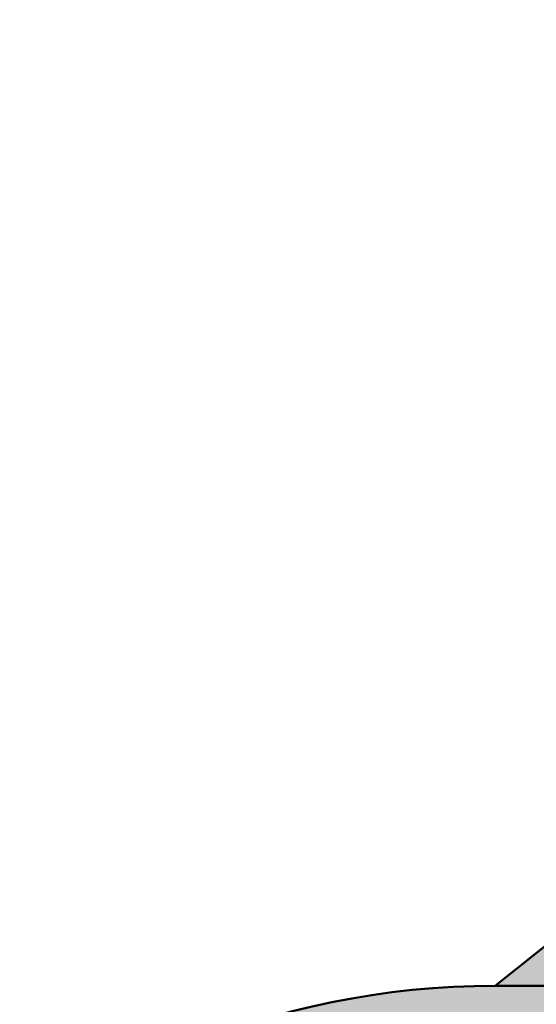
# Model space of a CAD drawing. Units: millimetres. Extents: x 0 to 2267, y 0 to 1823.
# Tile 17 of 256: x 1525.06 to 1531.44, y 1127.19 to 1139.34. Entities that reach past the tile are written whole.
import ezdxf

# ---------------------------------------------------------------- set-up
doc = ezdxf.new("R2010")
doc.units = ezdxf.units.MM
doc.header["$MEASUREMENT"] = 0
for name, color, linetype, lineweight in [('M-DIMS', 2, 'Continuous', 25), ('M-HATC', 252, 'Continuous', 18), ('M-OUTL', 7, 'Continuous', 50)]:
    doc.layers.add(name, color=color, linetype=linetype, lineweight=lineweight)
doc.styles.get("Standard").update_dxf_attribs({"font": 'arial.ttf'})
doc.dimstyles.get("Standard").update_dxf_attribs({"dimtxt": 7, "dimasz": 4, "dimexe": 0.18, "dimexo": 0.0625, "dimgap": 0.09, "dimtad": 0, "dimdec": 0, "dimzin": 0, "dimdsep": 46, "dimtxsty": 'Standard', "dimcen": 0.09, "dimadec": 0, "dimazin": 0, "dimtfac": 1, "dimtdec": 0, "dimtofl": 0, "dimtmove": 0, "dimatfit": 3, "dimfxl": 1, "dimtolj": 1, "dimtzin": 0, "dimarcsym": 0})

# ---------------------------------------------------------------- blocks, each defined once
blk = doc.blocks.new('*D28')
at = {"layer": 'Defpoints', "color": 0, "transparency": 16777216}
for p in [(1523.858, 1124.488), (1530.929, 1117.417)]:
    blk.add_point(p, dxfattribs=at)
at = {"layer": 'M-DIMS', "color": 0, "lineweight": -2, "transparency": 16777216}
for p, q in [((1518.201, 1130.145), (1521.029, 1127.317)), ((1530.929, 1117.327), (1530.929, 1117.507)), ((1530.839, 1117.417), (1531.019, 1117.417))]:
    blk.add_line(p, q, dxfattribs=at)
at = {"layer": 'M-DIMS', "color": 0, "transparency": 16777216}
blk.add_solid([(1521.501, 1127.788), (1520.558, 1126.845), (1523.858, 1124.488)], dxfattribs=at)
at = {"layer": 'M-DIMS', "color": 0, "transparency": 16777216, "insert": (1504.949, 1143.397), "char_height": 7, "attachment_point": 5, "rotation": 314.9998}
blk.add_mtext('\\A1;27X R10', dxfattribs=at)

msp = doc.modelspace()

# ---------------------------------------------------------------- hatches: boundary and pattern name
at = {"layer": 'M-HATC'}
h = msp.add_hatch(color=256, dxfattribs=at)
h.dxf.hatch_style = 1
h.paths.add_polyline_path([(2055.771, 1603.062), (1381.087, 1603.062), (1381.087, 1598.062), (2055.771, 1598.062)])
h.paths.add_polyline_path([(2055.771, 1598.062), (1381.087, 1598.062), (1381.087, 1593.062), (2055.771, 1593.062)])
h.paths.add_polyline_path([(2051.307, 1536.761), (1385.55, 1536.761), (1385.55, 1526.761), (1387.55, 1526.761), (1388.537, 1525.053), (1385.332, 1521.233), (1385.332, 1521.223), (2050.254, 1522.749), (2048.321, 1525.053), (2049.307, 1526.761), (2051.307, 1526.761)])
edge = h.paths.add_edge_path()
edge.add_arc((1847.535, 1379.149), 135, 222.60306, 222.89085, ccw=False)
edge.add_line((1748.166, 1287.766), (1683.092, 1287.766))
edge.add_arc((1583.724, 1379.149), 135, 317.10915, 317.39694, ccw=False)
edge.add_arc((1678.969, 1290.671), 5, 222.8909, 317.1091, ccw=False)
edge.add_arc((1774.213, 1379.149), 135, 222.60306, 222.89085, ccw=False)
edge.add_line((1674.845, 1287.766), (1609.771, 1287.766))
edge.add_arc((1510.403, 1379.149), 135, 317.10915, 317.39694, ccw=False)
edge.add_arc((1605.647, 1290.671), 5, 222.8909, 317.1091, ccw=False)
edge.add_arc((1700.892, 1379.149), 135, 222.60306, 222.89085, ccw=False)
edge.add_line((1601.524, 1287.766), (1536.45, 1287.766))
edge.add_arc((1437.081, 1379.149), 135, 317.10915, 317.39694, ccw=False)
edge.add_arc((1532.326, 1290.671), 5, 222.8909, 317.1091, ccw=False)
edge.add_arc((1627.571, 1379.149), 135, 222.60306, 222.89085, ccw=False)
edge.add_line((1528.203, 1287.766), (1505.929, 1287.766))
edge.add_spline(control_points=[(1505.929, 1287.766), (1504.262, 1287.766), (1504.262, 1282.766), (1505.929, 1282.766)], knot_values=[0, 0, 0, 0, 5, 5, 5, 5], degree=3, periodic=0)
edge.add_line((1505.929, 1282.766), (1930.929, 1282.766))
edge.add_spline(control_points=[(1930.929, 1282.766), (1932.596, 1282.766), (1932.596, 1287.766), (1930.929, 1287.766)], knot_values=[0, 0, 0, 0, 5, 5, 5, 5], degree=3, periodic=0)
edge.add_line((1930.929, 1287.766), (1903.056, 1287.766))
edge.add_arc((1803.688, 1379.149), 135, 317.10915, 317.39694, ccw=False)
edge.add_arc((1898.932, 1290.671), 5, 222.8909, 317.1091, ccw=False)
edge.add_arc((1994.177, 1379.149), 135, 222.60306, 222.89085, ccw=False)
edge.add_line((1894.809, 1287.766), (1829.735, 1287.766))
edge.add_arc((1730.366, 1379.149), 135, 317.10915, 317.39694, ccw=False)
edge.add_arc((1825.611, 1290.671), 5, 222.8909, 317.1091, ccw=False)
edge.add_arc((1920.856, 1379.149), 135, 222.60306, 222.89085, ccw=False)
edge.add_line((1821.487, 1287.766), (1756.413, 1287.766))
edge.add_arc((1657.045, 1379.149), 135, 317.10915, 317.39694, ccw=False)
edge.add_arc((1752.29, 1290.671), 5, 222.8909, 317.1091, ccw=False)
edge = h.paths.add_edge_path()
edge.add_spline(control_points=[(1843.429, 1227.247), (1845.096, 1227.247), (1845.096, 1232.247), (1843.429, 1232.247)], knot_values=[0, 0, 0, 0, 5, 5, 5, 5], degree=3, periodic=0)
edge.add_line((1843.429, 1232.247), (1593.429, 1232.247))
edge.add_spline(control_points=[(1593.429, 1232.247), (1591.762, 1232.247), (1591.762, 1227.247), (1593.429, 1227.247)], knot_values=[0, 0, 0, 0, 5, 5, 5, 5], degree=3, periodic=0)
edge.add_line((1593.429, 1227.247), (1843.429, 1227.247))
h.paths.add_polyline_path([(1905.929, 1127.417), (1530.929, 1127.417, 0.414214), (1520.929, 1117.417), (1530.929, 1117.417), (1915.929, 1117.417, 0.414214)])
edge = h.paths.add_edge_path()
edge.add_arc((1397.086, 1498.408), 12.73, 90.7821, 190.8787, ccw=False)
edge.add_line((1396.912, 1511.136), (1428.01, 1511.349))
edge.add_line((1428.01, 1511.349), (1433.01, 1511.349))
edge.add_line((1433.01, 1511.349), (1434.439, 1511.349))
edge.add_arc((1419.474, 1498.08), 20, 41.561, 74.0821)
edge.add_line((1424.959, 1517.314), (1399.935, 1517.256))
edge.add_spline(control_points=[(1399.931, 1517.256), (1399.884, 1517.213), (1399.833, 1517.169), (1399.777, 1517.124)], knot_values=[11.567499, 11.567499, 11.567499, 11.567499, 11.814249, 11.814249, 11.814249, 11.814249], degree=3, periodic=0)
edge.add_spline(control_points=[(1399.633, 1517.01), (1399.583, 1516.972), (1399.531, 1516.934), (1399.476, 1516.895)], knot_values=[11.167718, 11.167718, 11.167718, 11.167718, 11.365188, 11.365188, 11.365188, 11.365188], degree=3, periodic=0)
edge.add_spline(control_points=[(1399.34, 1516.8), (1399.151, 1516.672), (1398.938, 1516.538), (1398.704, 1516.399)], knot_values=[10.376405, 10.376405, 10.376405, 10.376405, 11.00994, 11.00994, 11.00994, 11.00994], degree=3, periodic=0)
edge.add_spline(control_points=[(1398.657, 1516.372), (1398.579, 1516.326), (1398.498, 1516.28), (1398.415, 1516.233)], knot_values=[10.125175, 10.125175, 10.125175, 10.125175, 10.334406, 10.334406, 10.334406, 10.334406], degree=3, periodic=0)
edge.add_spline(control_points=[(1398.264, 1516.149), (1398.196, 1516.111), (1398.126, 1516.073), (1398.055, 1516.035)], knot_values=[9.832246, 9.832246, 9.832246, 9.832246, 9.999658, 9.999658, 9.999658, 9.999658], degree=3, periodic=0)
edge.add_spline(control_points=[(1397.999, 1516.005), (1397.731, 1515.862), (1397.446, 1515.717), (1397.147, 1515.571)], knot_values=[9.161808, 9.161808, 9.161808, 9.161808, 9.787769, 9.787769, 9.787769, 9.787769], degree=3, periodic=0)
edge.add_spline(control_points=[(1397.147, 1515.571), (1396.842, 1515.423), (1396.522, 1515.274), (1396.191, 1515.126)], knot_values=[8.524455, 8.524455, 8.524455, 8.524455, 9.161808, 9.161808, 9.161808, 9.161808], degree=3, periodic=0)
edge.add_spline(control_points=[(1396.078, 1515.076), (1395.985, 1515.035), (1395.892, 1514.994), (1395.798, 1514.953)], knot_values=[8.275193, 8.275193, 8.275193, 8.275193, 8.451726, 8.451726, 8.451726, 8.451726], degree=3, periodic=0)
edge.add_spline(control_points=[(1395.602, 1514.869), (1395.5, 1514.826), (1395.397, 1514.782), (1395.293, 1514.739)], knot_values=[7.962917, 7.962917, 7.962917, 7.962917, 8.152764, 8.152764, 8.152764, 8.152764], degree=3, periodic=0)
edge.add_spline(control_points=[(1395.212, 1514.706), (1394.828, 1514.547), (1394.435, 1514.393), (1394.036, 1514.244)], knot_values=[7.21254, 7.21254, 7.21254, 7.21254, 7.913148, 7.913148, 7.913148, 7.913148], degree=3, periodic=0)
edge.add_spline(control_points=[(1394.036, 1514.244), (1393.708, 1514.121), (1393.375, 1514.003), (1393.043, 1513.889)], knot_values=[6.633733, 6.633733, 6.633733, 6.633733, 7.21254, 7.21254, 7.21254, 7.21254], degree=3, periodic=0)
edge.add_spline(control_points=[(1392.821, 1513.815), (1392.72, 1513.781), (1392.618, 1513.748), (1392.517, 1513.715)], knot_values=[6.328796, 6.328796, 6.328796, 6.328796, 6.505493, 6.505493, 6.505493, 6.505493], degree=3, periodic=0)
edge.add_spline(control_points=[(1392.517, 1513.715), (1392.319, 1513.652), (1392.121, 1513.59), (1391.924, 1513.531)], knot_values=[5.984605, 5.984605, 5.984605, 5.984605, 6.328796, 6.328796, 6.328796, 6.328796], degree=3, periodic=0)
edge.add_spline(control_points=[(1391.792, 1513.491), (1391.312, 1513.35), (1390.838, 1513.224), (1390.378, 1513.117)], knot_values=[5.066697, 5.066697, 5.066697, 5.066697, 5.907055, 5.907055, 5.907055, 5.907055], degree=3, periodic=0)
edge.add_spline(control_points=[(1390.378, 1513.117), (1390.18, 1513.071), (1389.984, 1513.028), (1389.791, 1512.99)], knot_values=[4.70367, 4.70367, 4.70367, 4.70367, 5.066695, 5.066695, 5.066695, 5.066695], degree=3, periodic=0)
edge.add_spline(control_points=[(1389.422, 1512.92), (1389.246, 1512.889), (1389.073, 1512.862), (1388.904, 1512.838)], knot_values=[4.130571, 4.130571, 4.130571, 4.130571, 4.469816, 4.469816, 4.469816, 4.469816], degree=3, periodic=0)
edge.add_spline(control_points=[(1388.904, 1512.838), (1388.591, 1512.795), (1388.291, 1512.764), (1388.007, 1512.749)], knot_values=[3.504031, 3.504031, 3.504031, 3.504031, 4.130571, 4.130571, 4.130571, 4.130571], degree=3, periodic=0)
edge.add_spline(control_points=[(1387.936, 1512.746), (1387.854, 1512.742), (1387.773, 1512.74), (1387.694, 1512.739)], knot_values=[3.268866, 3.268866, 3.268866, 3.268866, 3.451164, 3.451164, 3.451164, 3.451164], degree=3, periodic=0)
edge.add_spline(control_points=[(1387.335, 1512.744), (1387.208, 1512.75), (1387.085, 1512.76), (1386.967, 1512.774)], knot_values=[2.670686, 2.670686, 2.670686, 2.670686, 2.984, 2.984, 2.984, 2.984], degree=3, periodic=0)
edge.add_spline(control_points=[(1386.833, 1512.792), (1386.821, 1512.794), (1386.809, 1512.796), (1386.797, 1512.798)], knot_values=[2.516981, 2.516981, 2.516981, 2.516981, 2.549528, 2.549528, 2.549528, 2.549528], degree=3, periodic=0)
edge.add_spline(control_points=[(1386.453, 1512.873), (1386.426, 1512.881), (1386.399, 1512.889), (1386.373, 1512.897)], knot_values=[2.095869, 2.095869, 2.095869, 2.095869, 2.17941, 2.17941, 2.17941, 2.17941], degree=3, periodic=0)
edge.add_spline(control_points=[(1386.069, 1513.019), (1386.063, 1513.022), (1386.058, 1513.025), (1386.052, 1513.028)], knot_values=[1.72453, 1.72453, 1.72453, 1.72453, 1.745933, 1.745933, 1.745933, 1.745933], degree=3, periodic=0)
edge.add_arc((1399.474, 1498.08), 20, 131.8243, 180)
edge.add_arc((1630.334, 1505.548), 250.971, 181.70518, 236.42798)
edge.add_arc((1605.34, 1483.304), 218.782, 238.66083, 243.34961)
edge.add_arc((1647.091, 1510.359), 262.899, 183.12984, 237.85344, ccw=False)
h.paths.add_polyline_path([(1406.537, 1391.964, 0.149382), (1491.551, 1296.442, -0.129517)], flags=17)
edge = h.paths.add_edge_path()
edge.add_arc((2037.384, 1498.08), 20, 0, 48.2659)
edge.add_spline(control_points=[(2050.697, 1513.005), (2050.651, 1512.985), (2050.603, 1512.966), (2050.554, 1512.948)], knot_values=[1.835652, 1.835652, 1.835652, 1.835652, 2.000781, 2.000781, 2.000781, 2.000781], degree=3, periodic=0)
edge.add_spline(control_points=[(2050.462, 1512.917), (2050.479, 1512.922), (2050.496, 1512.928), (2050.513, 1512.934)], knot_values=[2.045477, 2.045477, 2.045477, 2.045477, 2.101389, 2.101389, 2.101389, 2.101389], degree=3, periodic=0)
edge.add_spline(control_points=[(2050.129, 1512.834), (2050.198, 1512.847), (2050.266, 1512.862), (2050.331, 1512.879)], knot_values=[2.237629, 2.237629, 2.237629, 2.237629, 2.435841, 2.435841, 2.435841, 2.435841], degree=3, periodic=0)
edge.add_spline(control_points=[(2050.095, 1512.828), (2050.106, 1512.83), (2050.118, 1512.832), (2050.129, 1512.834)], knot_values=[2.435841, 2.435841, 2.435841, 2.435841, 2.468321, 2.468321, 2.468321, 2.468321], degree=3, periodic=0)
edge.add_spline(control_points=[(2049.784, 1512.785), (2049.855, 1512.792), (2049.924, 1512.801), (2049.992, 1512.811)], knot_values=[2.563852, 2.563852, 2.563852, 2.563852, 2.748541, 2.748541, 2.748541, 2.748541], degree=3, periodic=0)
edge.add_spline(control_points=[(2049.405, 1512.762), (2049.536, 1512.765), (2049.663, 1512.773), (2049.784, 1512.785)], knot_values=[2.748541, 2.748541, 2.748541, 2.748541, 3.064882, 3.064882, 3.064882, 3.064882], degree=3, periodic=0)
edge.add_spline(control_points=[(2049.17, 1512.76), (2049.234, 1512.759), (2049.297, 1512.759), (2049.358, 1512.761)], knot_values=[3.102309, 3.102309, 3.102309, 3.102309, 3.2503, 3.2503, 3.2503, 3.2503], degree=3, periodic=0)
edge.add_spline(control_points=[(2048.857, 1512.769), (2048.964, 1512.764), (2049.068, 1512.761), (2049.17, 1512.76)], knot_values=[3.2503, 3.2503, 3.2503, 3.2503, 3.486069, 3.486069, 3.486069, 3.486069], degree=3, periodic=0)
edge.add_spline(control_points=[(2048.692, 1512.779), (2048.373, 1512.801), (2048.035, 1512.841), (2047.682, 1512.897)], knot_values=[3.606429, 3.606429, 3.606429, 3.606429, 4.2989, 4.2989, 4.2989, 4.2989], degree=3, periodic=0)
edge.add_spline(control_points=[(2047.682, 1512.897), (2047.546, 1512.919), (2047.408, 1512.942), (2047.268, 1512.969)], knot_values=[4.2989, 4.2989, 4.2989, 4.2989, 4.565769, 4.565769, 4.565769, 4.565769], degree=3, periodic=0)
edge.add_spline(control_points=[(2047.268, 1512.969), (2047.145, 1512.991), (2047.021, 1513.016), (2046.895, 1513.042)], knot_values=[4.565769, 4.565769, 4.565769, 4.565769, 4.799971, 4.799971, 4.799971, 4.799971], degree=3, periodic=0)
edge.add_spline(control_points=[(2046.895, 1513.042), (2046.529, 1513.119), (2046.151, 1513.209), (2045.768, 1513.311)], knot_values=[4.799971, 4.799971, 4.799971, 4.799971, 5.483718, 5.483718, 5.483718, 5.483718], degree=3, periodic=0)
edge.add_spline(control_points=[(2045.768, 1513.311), (2045.372, 1513.415), (2044.97, 1513.532), (2044.566, 1513.659)], knot_values=[5.483718, 5.483718, 5.483718, 5.483718, 6.187866, 6.187866, 6.187866, 6.187866], degree=3, periodic=0)
edge.add_spline(control_points=[(2044.566, 1513.659), (2044.415, 1513.706), (2044.263, 1513.755), (2044.112, 1513.805)], knot_values=[6.187866, 6.187866, 6.187866, 6.187866, 6.451551, 6.451551, 6.451551, 6.451551], degree=3, periodic=0)
edge.add_spline(control_points=[(2044.112, 1513.805), (2043.997, 1513.843), (2043.882, 1513.881), (2043.767, 1513.92)], knot_values=[6.451551, 6.451551, 6.451551, 6.451551, 6.651434, 6.651434, 6.651434, 6.651434], degree=3, periodic=0)
edge.add_spline(control_points=[(2043.767, 1513.92), (2043.372, 1514.055), (2042.977, 1514.198), (2042.589, 1514.346)], knot_values=[6.651434, 6.651434, 6.651434, 6.651434, 7.338879, 7.338879, 7.338879, 7.338879], degree=3, periodic=0)
edge.add_spline(control_points=[(2042.589, 1514.346), (2042.164, 1514.507), (2041.746, 1514.675), (2041.341, 1514.846)], knot_values=[7.338879, 7.338879, 7.338879, 7.338879, 8.089209, 8.089209, 8.089209, 8.089209], degree=3, periodic=0)
edge.add_spline(control_points=[(2041.341, 1514.846), (2041.103, 1514.946), (2040.869, 1515.048), (2040.64, 1515.15)], knot_values=[8.089209, 8.089209, 8.089209, 8.089209, 8.529587, 8.529587, 8.529587, 8.529587], degree=3, periodic=0)
edge.add_spline(control_points=[(2040.51, 1515.209), (2040.082, 1515.402), (2039.675, 1515.597), (2039.295, 1515.789)], knot_values=[8.613818, 8.613818, 8.613818, 8.613818, 9.44571, 9.44571, 9.44571, 9.44571], degree=3, periodic=0)
edge.add_spline(control_points=[(2039.295, 1515.789), (2039.062, 1515.907), (2038.839, 1516.025), (2038.629, 1516.14)], knot_values=[9.44571, 9.44571, 9.44571, 9.44571, 9.956404, 9.956404, 9.956404, 9.956404], degree=3, periodic=0)
edge.add_spline(control_points=[(2038.629, 1516.14), (2038.519, 1516.2), (2038.412, 1516.26), (2038.309, 1516.319)], knot_values=[9.956404, 9.956404, 9.956404, 9.956404, 10.223542, 10.223542, 10.223542, 10.223542], degree=3, periodic=0)
edge.add_spline(control_points=[(2038.309, 1516.319), (2038.214, 1516.374), (2038.122, 1516.428), (2038.033, 1516.481)], knot_values=[10.223542, 10.223542, 10.223542, 10.223542, 10.47051, 10.47051, 10.47051, 10.47051], degree=3, periodic=0)
edge.add_spline(control_points=[(2038.033, 1516.481), (2037.786, 1516.63), (2037.564, 1516.773), (2037.372, 1516.909)], knot_values=[10.47051, 10.47051, 10.47051, 10.47051, 11.15767, 11.15767, 11.15767, 11.15767], degree=3, periodic=0)
edge.add_spline(control_points=[(2037.372, 1516.909), (2037.279, 1516.975), (2037.193, 1517.04), (2037.114, 1517.102)], knot_values=[11.15767, 11.15767, 11.15767, 11.15767, 11.49227, 11.49227, 11.49227, 11.49227], degree=3, periodic=0)
edge.add_spline(control_points=[(2036.856, 1517.326), (2036.915, 1517.269), (2036.981, 1517.21), (2037.056, 1517.149)], knot_values=[11.577341, 11.577341, 11.577341, 11.577341, 11.91035, 11.91035, 11.91035, 11.91035], degree=3, periodic=0)
edge.add_spline(control_points=[(2036.807, 1517.375), (2036.823, 1517.359), (2036.839, 1517.342), (2036.856, 1517.326)], knot_values=[11.91035, 11.91035, 11.91035, 11.91035, 12.007402, 12.007402, 12.007402, 12.007402], degree=3, periodic=0)
edge.add_spline(control_points=[(2036.702, 1517.494), (2036.71, 1517.483), (2036.72, 1517.472), (2036.729, 1517.461)], knot_values=[12.184155, 12.184155, 12.184155, 12.184155, 12.255409, 12.255409, 12.255409, 12.255409], degree=3, periodic=0)
edge.add_spline(control_points=[(2036.616, 1517.621), (2036.62, 1517.613), (2036.624, 1517.606), (2036.629, 1517.598)], knot_values=[12.487913, 12.487913, 12.487913, 12.487913, 12.541035, 12.541035, 12.541035, 12.541035], degree=3, periodic=0)
edge.add_spline(control_points=[(2036.563, 1517.786), (2036.564, 1517.779), (2036.564, 1517.773), (2036.565, 1517.766)], knot_values=[12.911761, 12.911761, 12.911761, 12.911761, 12.968286, 12.968286, 12.968286, 12.968286], degree=3, periodic=0)
edge.add_spline(control_points=[(2036.617, 1517.93), (2036.612, 1517.926), (2036.609, 1517.921), (2036.605, 1517.916)], knot_values=[13.382527, 13.382527, 13.382527, 13.382527, 13.433791, 13.433791, 13.433791, 13.433791], degree=3, periodic=0)
edge.add_spline(control_points=[(2036.749, 1518.017), (2036.736, 1518.012), (2036.724, 1518.006), (2036.712, 1518)], knot_values=[13.726299, 13.726299, 13.726299, 13.726299, 13.809928, 13.809928, 13.809928, 13.809928], degree=3, periodic=0)
edge.add_spline(control_points=[(2036.86, 1518.053), (2036.839, 1518.047), (2036.818, 1518.042), (2036.799, 1518.035)], knot_values=[13.910887, 13.910887, 13.910887, 13.910887, 14.02153, 14.02153, 14.02153, 14.02153], degree=3, periodic=0)
edge.add_line((2036.964, 1518.08), (2032.384, 1518.08))
edge.add_line((2032.384, 1518.08), (2027.384, 1518.08))
edge.add_line((2027.384, 1518.08), (2022.384, 1518.08))
edge.add_line((2022.384, 1518.08), (2017.384, 1518.08))
edge.add_arc((2017.384, 1498.08), 20, 90, 138.439)
edge.add_line((2002.419, 1511.349), (2003.848, 1511.349))
edge.add_line((2003.848, 1511.349), (2008.848, 1511.349))
edge.add_line((2008.848, 1511.349), (2039.772, 1511.138))
edge.add_arc((2039.772, 1498.408), 12.73, -10.8787, 90, ccw=False)
edge.add_arc((1789.767, 1510.359), 262.899, 302.14656, 356.87016, ccw=False)
edge.add_arc((1831.518, 1483.304), 218.782, 296.65039, 301.33917)
edge.add_arc((1806.524, 1505.548), 250.971, 303.57202, 358.29482)
h.paths.add_polyline_path([(2030.321, 1391.964, -0.129517), (1945.307, 1296.442, 0.149382)], flags=17)
edge = h.paths.add_edge_path()
edge.add_spline(control_points=[(2037.246, 1518.082), (2037.29, 1518.081), (2037.336, 1518.08), (2037.384, 1518.08)], knot_values=[0.000012, 0.000012, 0.000012, 0.000012, 0.144754, 0.144754, 0.144754, 0.144754], degree=3, periodic=0)
edge.add_line((2037.336, 1518.08), (2037.01, 1518.08))
edge.add_spline(control_points=[(2037.01, 1518.08), (2036.982, 1518.077), (2036.956, 1518.073), (2036.931, 1518.068)], knot_values=[14.13465, 14.13465, 14.13465, 14.13465, 14.247197, 14.247197, 14.247197, 14.247197], degree=3, periodic=0)
edge.add_spline(control_points=[(2036.931, 1518.068), (2036.928, 1518.067), (2036.924, 1518.067), (2036.921, 1518.066)], knot_values=[14.118315, 14.118315, 14.118315, 14.118315, 14.13465, 14.13465, 14.13465, 14.13465], degree=3, periodic=0)
edge.add_spline(control_points=[(2036.921, 1518.066), (2036.912, 1518.064), (2036.903, 1518.063), (2036.895, 1518.061)], knot_values=[14.078086, 14.078086, 14.078086, 14.078086, 14.118315, 14.118315, 14.118315, 14.118315], degree=3, periodic=0)
edge.add_spline(control_points=[(2036.895, 1518.061), (2036.883, 1518.058), (2036.872, 1518.056), (2036.86, 1518.053)], knot_values=[14.02153, 14.02153, 14.02153, 14.02153, 14.078086, 14.078086, 14.078086, 14.078086], degree=3, periodic=0)
edge.add_spline(control_points=[(2036.86, 1518.053), (2036.839, 1518.047), (2036.818, 1518.042), (2036.799, 1518.035)], knot_values=[13.910887, 13.910887, 13.910887, 13.910887, 14.02153, 14.02153, 14.02153, 14.02153], degree=3, periodic=0)
edge.add_spline(control_points=[(2036.799, 1518.035), (2036.798, 1518.035), (2036.797, 1518.035), (2036.797, 1518.035)], knot_values=[13.906906, 13.906906, 13.906906, 13.906906, 13.910887, 13.910887, 13.910887, 13.910887], degree=3, periodic=0)
edge.add_spline(control_points=[(2036.797, 1518.035), (2036.788, 1518.032), (2036.78, 1518.029), (2036.772, 1518.026)], knot_values=[13.857826, 13.857826, 13.857826, 13.857826, 13.906906, 13.906906, 13.906906, 13.906906], degree=3, periodic=0)
edge.add_spline(control_points=[(2036.772, 1518.026), (2036.764, 1518.023), (2036.756, 1518.02), (2036.749, 1518.017)], knot_values=[13.809928, 13.809928, 13.809928, 13.809928, 13.857826, 13.857826, 13.857826, 13.857826], degree=3, periodic=0)
edge.add_spline(control_points=[(2036.749, 1518.017), (2036.736, 1518.012), (2036.724, 1518.006), (2036.712, 1518)], knot_values=[13.726299, 13.726299, 13.726299, 13.726299, 13.809928, 13.809928, 13.809928, 13.809928], degree=3, periodic=0)
edge.add_spline(control_points=[(2036.712, 1518), (2036.712, 1518), (2036.712, 1518), (2036.711, 1518)], knot_values=[13.723993, 13.723993, 13.723993, 13.723993, 13.726299, 13.726299, 13.726299, 13.726299], degree=3, periodic=0)
edge.add_spline(control_points=[(2036.711, 1518), (2036.706, 1517.997), (2036.701, 1517.994), (2036.696, 1517.992)], knot_values=[13.686536, 13.686536, 13.686536, 13.686536, 13.723993, 13.723993, 13.723993, 13.723993], degree=3, periodic=0)
edge.add_spline(control_points=[(2036.696, 1517.992), (2036.692, 1517.989), (2036.687, 1517.987), (2036.683, 1517.984)], knot_values=[13.651251, 13.651251, 13.651251, 13.651251, 13.686536, 13.686536, 13.686536, 13.686536], degree=3, periodic=0)
edge.add_spline(control_points=[(2036.683, 1517.984), (2036.676, 1517.98), (2036.67, 1517.976), (2036.664, 1517.971)], knot_values=[13.596804, 13.596804, 13.596804, 13.596804, 13.651251, 13.651251, 13.651251, 13.651251], degree=3, periodic=0)
edge.add_spline(control_points=[(2036.664, 1517.971), (2036.664, 1517.971), (2036.663, 1517.971), (2036.663, 1517.971)], knot_values=[13.593956, 13.593956, 13.593956, 13.593956, 13.596804, 13.596804, 13.596804, 13.596804], degree=3, periodic=0)
edge.add_spline(control_points=[(2036.663, 1517.971), (2036.66, 1517.969), (2036.658, 1517.967), (2036.655, 1517.965)], knot_values=[13.570322, 13.570322, 13.570322, 13.570322, 13.593956, 13.593956, 13.593956, 13.593956], degree=3, periodic=0)
edge.add_spline(control_points=[(2036.655, 1517.965), (2036.653, 1517.963), (2036.65, 1517.961), (2036.647, 1517.959)], knot_values=[13.545477, 13.545477, 13.545477, 13.545477, 13.570322, 13.570322, 13.570322, 13.570322], degree=3, periodic=0)
edge.add_spline(control_points=[(2036.647, 1517.959), (2036.647, 1517.959), (2036.647, 1517.959), (2036.647, 1517.959)], knot_values=[13.543931, 13.543931, 13.543931, 13.543931, 13.545477, 13.545477, 13.545477, 13.545477], degree=3, periodic=0)
edge.add_spline(control_points=[(2036.647, 1517.959), (2036.641, 1517.954), (2036.636, 1517.949), (2036.631, 1517.945)], knot_values=[13.488237, 13.488237, 13.488237, 13.488237, 13.543931, 13.543931, 13.543931, 13.543931], degree=3, periodic=0)
edge.add_spline(control_points=[(2036.631, 1517.945), (2036.628, 1517.942), (2036.626, 1517.94), (2036.623, 1517.937)], knot_values=[13.460307, 13.460307, 13.460307, 13.460307, 13.488237, 13.488237, 13.488237, 13.488237], degree=3, periodic=0)
edge.add_spline(control_points=[(2036.623, 1517.937), (2036.622, 1517.936), (2036.62, 1517.934), (2036.618, 1517.932)], knot_values=[13.439712, 13.439712, 13.439712, 13.439712, 13.460307, 13.460307, 13.460307, 13.460307], degree=3, periodic=0)
edge.add_spline(control_points=[(2036.618, 1517.932), (2036.618, 1517.931), (2036.617, 1517.931), (2036.617, 1517.93)], knot_values=[13.433791, 13.433791, 13.433791, 13.433791, 13.439712, 13.439712, 13.439712, 13.439712], degree=3, periodic=0)
edge.add_spline(control_points=[(2036.617, 1517.93), (2036.612, 1517.926), (2036.609, 1517.921), (2036.605, 1517.916)], knot_values=[13.382527, 13.382527, 13.382527, 13.382527, 13.433791, 13.433791, 13.433791, 13.433791], degree=3, periodic=0)
edge.add_spline(control_points=[(2036.605, 1517.916), (2036.603, 1517.913), (2036.6, 1517.91), (2036.598, 1517.907)], knot_values=[13.350017, 13.350017, 13.350017, 13.350017, 13.382527, 13.382527, 13.382527, 13.382527], degree=3, periodic=0)
edge.add_spline(control_points=[(2036.598, 1517.907), (2036.597, 1517.906), (2036.596, 1517.904), (2036.595, 1517.903)], knot_values=[13.333922, 13.333922, 13.333922, 13.333922, 13.350017, 13.350017, 13.350017, 13.350017], degree=3, periodic=0)
edge.add_spline(control_points=[(2036.595, 1517.903), (2036.595, 1517.902), (2036.594, 1517.901), (2036.593, 1517.9)], knot_values=[13.323828, 13.323828, 13.323828, 13.323828, 13.333922, 13.333922, 13.333922, 13.333922], degree=3, periodic=0)
edge.add_spline(control_points=[(2036.593, 1517.9), (2036.59, 1517.895), (2036.588, 1517.891), (2036.585, 1517.886)], knot_values=[13.277545, 13.277545, 13.277545, 13.277545, 13.323828, 13.323828, 13.323828, 13.323828], degree=3, periodic=0)
edge.add_spline(control_points=[(2036.585, 1517.886), (2036.584, 1517.883), (2036.582, 1517.879), (2036.58, 1517.875)], knot_values=[13.240119, 13.240119, 13.240119, 13.240119, 13.277545, 13.277545, 13.277545, 13.277545], degree=3, periodic=0)
edge.add_spline(control_points=[(2036.58, 1517.875), (2036.58, 1517.874), (2036.579, 1517.873), (2036.578, 1517.872)], knot_values=[13.228211, 13.228211, 13.228211, 13.228211, 13.240119, 13.240119, 13.240119, 13.240119], degree=3, periodic=0)
edge.add_spline(control_points=[(2036.578, 1517.872), (2036.578, 1517.87), (2036.577, 1517.869), (2036.577, 1517.868)], knot_values=[13.215717, 13.215717, 13.215717, 13.215717, 13.228211, 13.228211, 13.228211, 13.228211], degree=3, periodic=0)
edge.add_spline(control_points=[(2036.577, 1517.868), (2036.575, 1517.864), (2036.574, 1517.86), (2036.573, 1517.857)], knot_values=[13.179847, 13.179847, 13.179847, 13.179847, 13.215717, 13.215717, 13.215717, 13.215717], degree=3, periodic=0)
edge.add_spline(control_points=[(2036.573, 1517.857), (2036.571, 1517.851), (2036.57, 1517.846), (2036.569, 1517.841)], knot_values=[13.132017, 13.132017, 13.132017, 13.132017, 13.179847, 13.179847, 13.179847, 13.179847], degree=3, periodic=0)
edge.add_spline(control_points=[(2036.569, 1517.841), (2036.568, 1517.84), (2036.568, 1517.839), (2036.568, 1517.838)], knot_values=[13.122482, 13.122482, 13.122482, 13.122482, 13.132017, 13.132017, 13.132017, 13.132017], degree=3, periodic=0)
edge.add_spline(control_points=[(2036.568, 1517.838), (2036.568, 1517.836), (2036.567, 1517.835), (2036.567, 1517.833)], knot_values=[13.105592, 13.105592, 13.105592, 13.105592, 13.122482, 13.122482, 13.122482, 13.122482], degree=3, periodic=0)
edge.add_spline(control_points=[(2036.567, 1517.833), (2036.566, 1517.829), (2036.566, 1517.826), (2036.565, 1517.822)], knot_values=[13.074063, 13.074063, 13.074063, 13.074063, 13.105592, 13.105592, 13.105592, 13.105592], degree=3, periodic=0)
edge.add_spline(control_points=[(2036.565, 1517.822), (2036.565, 1517.822), (2036.565, 1517.822), (2036.565, 1517.822)], knot_values=[13.074043, 13.074043, 13.074043, 13.074043, 13.074063, 13.074063, 13.074063, 13.074063], degree=3, periodic=0)
edge.add_spline(control_points=[(2036.565, 1517.822), (2036.564, 1517.816), (2036.564, 1517.811), (2036.564, 1517.805)], knot_values=[13.021884, 13.021884, 13.021884, 13.021884, 13.074043, 13.074043, 13.074043, 13.074043], degree=3, periodic=0)
edge.add_spline(control_points=[(2036.564, 1517.805), (2036.564, 1517.804), (2036.564, 1517.803), (2036.564, 1517.803)], knot_values=[13.01674, 13.01674, 13.01674, 13.01674, 13.021884, 13.021884, 13.021884, 13.021884], degree=3, periodic=0)
edge.add_spline(control_points=[(2036.564, 1517.803), (2036.563, 1517.801), (2036.563, 1517.798), (2036.563, 1517.796)], knot_values=[12.996438, 12.996438, 12.996438, 12.996438, 13.01674, 13.01674, 13.01674, 13.01674], degree=3, periodic=0)
edge.add_spline(control_points=[(2036.563, 1517.796), (2036.563, 1517.793), (2036.563, 1517.789), (2036.563, 1517.786)], knot_values=[12.968286, 12.968286, 12.968286, 12.968286, 12.996438, 12.996438, 12.996438, 12.996438], degree=3, periodic=0)
edge.add_spline(control_points=[(2036.563, 1517.786), (2036.564, 1517.779), (2036.564, 1517.773), (2036.565, 1517.766)], knot_values=[12.911761, 12.911761, 12.911761, 12.911761, 12.968286, 12.968286, 12.968286, 12.968286], degree=3, periodic=0)
edge.add_spline(control_points=[(2036.565, 1517.766), (2036.565, 1517.766), (2036.565, 1517.766), (2036.565, 1517.766)], knot_values=[12.911017, 12.911017, 12.911017, 12.911017, 12.911761, 12.911761, 12.911761, 12.911761], degree=3, periodic=0)
edge.add_spline(control_points=[(2036.565, 1517.766), (2036.565, 1517.762), (2036.566, 1517.759), (2036.566, 1517.756)], knot_values=[12.88528, 12.88528, 12.88528, 12.88528, 12.911017, 12.911017, 12.911017, 12.911017], degree=3, periodic=0)
edge.add_spline(control_points=[(2036.566, 1517.756), (2036.567, 1517.753), (2036.567, 1517.751), (2036.568, 1517.748)], knot_values=[12.862519, 12.862519, 12.862519, 12.862519, 12.88528, 12.88528, 12.88528, 12.88528], degree=3, periodic=0)
edge.add_spline(control_points=[(2036.568, 1517.748), (2036.568, 1517.747), (2036.568, 1517.747), (2036.568, 1517.746)], knot_values=[12.858885, 12.858885, 12.858885, 12.858885, 12.862519, 12.862519, 12.862519, 12.862519], degree=3, periodic=0)
edge.add_spline(control_points=[(2036.568, 1517.746), (2036.569, 1517.74), (2036.571, 1517.733), (2036.572, 1517.726)], knot_values=[12.8053, 12.8053, 12.8053, 12.8053, 12.858885, 12.858885, 12.858885, 12.858885], degree=3, periodic=0)
edge.add_spline(control_points=[(2036.572, 1517.726), (2036.573, 1517.723), (2036.574, 1517.719), (2036.576, 1517.715)], knot_values=[12.775176, 12.775176, 12.775176, 12.775176, 12.8053, 12.8053, 12.8053, 12.8053], degree=3, periodic=0)
edge.add_spline(control_points=[(2036.576, 1517.715), (2036.576, 1517.713), (2036.577, 1517.71), (2036.578, 1517.708)], knot_values=[12.756759, 12.756759, 12.756759, 12.756759, 12.775176, 12.775176, 12.775176, 12.775176], degree=3, periodic=0)
edge.add_spline(control_points=[(2036.578, 1517.708), (2036.578, 1517.707), (2036.578, 1517.706), (2036.579, 1517.705)], knot_values=[12.748742, 12.748742, 12.748742, 12.748742, 12.756759, 12.756759, 12.756759, 12.756759], degree=3, periodic=0)
edge.add_spline(control_points=[(2036.579, 1517.705), (2036.581, 1517.698), (2036.583, 1517.692), (2036.586, 1517.685)], knot_values=[12.69959, 12.69959, 12.69959, 12.69959, 12.748742, 12.748742, 12.748742, 12.748742], degree=3, periodic=0)
edge.add_spline(control_points=[(2036.586, 1517.685), (2036.588, 1517.68), (2036.59, 1517.675), (2036.592, 1517.669)], knot_values=[12.659038, 12.659038, 12.659038, 12.659038, 12.69959, 12.69959, 12.69959, 12.69959], degree=3, periodic=0)
edge.add_spline(control_points=[(2036.592, 1517.669), (2036.594, 1517.665), (2036.596, 1517.66), (2036.598, 1517.656)], knot_values=[12.626806, 12.626806, 12.626806, 12.626806, 12.659038, 12.659038, 12.659038, 12.659038], degree=3, periodic=0)
edge.add_spline(control_points=[(2036.598, 1517.656), (2036.598, 1517.655), (2036.599, 1517.654), (2036.599, 1517.653)], knot_values=[12.619394, 12.619394, 12.619394, 12.619394, 12.626806, 12.626806, 12.626806, 12.626806], degree=3, periodic=0)
edge.add_spline(control_points=[(2036.599, 1517.653), (2036.604, 1517.642), (2036.61, 1517.632), (2036.616, 1517.621)], knot_values=[12.541039, 12.541039, 12.541039, 12.541039, 12.619394, 12.619394, 12.619394, 12.619394], degree=3, periodic=0)
edge.add_spline(control_points=[(2036.616, 1517.621), (2036.616, 1517.621), (2036.616, 1517.621), (2036.616, 1517.621)], knot_values=[12.541035, 12.541035, 12.541035, 12.541035, 12.541039, 12.541039, 12.541039, 12.541039], degree=3, periodic=0)
edge.add_spline(control_points=[(2036.616, 1517.621), (2036.62, 1517.613), (2036.624, 1517.606), (2036.629, 1517.598)], knot_values=[12.487913, 12.487913, 12.487913, 12.487913, 12.541035, 12.541035, 12.541035, 12.541035], degree=3, periodic=0)
edge.add_spline(control_points=[(2036.629, 1517.598), (2036.633, 1517.592), (2036.637, 1517.585), (2036.641, 1517.579)], knot_values=[12.443982, 12.443982, 12.443982, 12.443982, 12.487913, 12.487913, 12.487913, 12.487913], degree=3, periodic=0)
edge.add_spline(control_points=[(2036.641, 1517.579), (2036.641, 1517.578), (2036.642, 1517.576), (2036.643, 1517.575)], knot_values=[12.434996, 12.434996, 12.434996, 12.434996, 12.443982, 12.443982, 12.443982, 12.443982], degree=3, periodic=0)
edge.add_spline(control_points=[(2036.643, 1517.575), (2036.653, 1517.56), (2036.664, 1517.544), (2036.676, 1517.528)], knot_values=[12.329647, 12.329647, 12.329647, 12.329647, 12.434996, 12.434996, 12.434996, 12.434996], degree=3, periodic=0)
edge.add_spline(control_points=[(2036.676, 1517.528), (2036.684, 1517.517), (2036.693, 1517.505), (2036.702, 1517.494)], knot_values=[12.255409, 12.255409, 12.255409, 12.255409, 12.329647, 12.329647, 12.329647, 12.329647], degree=3, periodic=0)
edge.add_spline(control_points=[(2036.702, 1517.494), (2036.71, 1517.483), (2036.72, 1517.472), (2036.729, 1517.461)], knot_values=[12.184155, 12.184155, 12.184155, 12.184155, 12.255409, 12.255409, 12.255409, 12.255409], degree=3, periodic=0)
edge.add_spline(control_points=[(2036.729, 1517.461), (2036.744, 1517.444), (2036.759, 1517.426), (2036.775, 1517.409)], knot_values=[12.075961, 12.075961, 12.075961, 12.075961, 12.184155, 12.184155, 12.184155, 12.184155], degree=3, periodic=0)
edge.add_spline(control_points=[(2036.775, 1517.409), (2036.776, 1517.407), (2036.777, 1517.406), (2036.778, 1517.405)], knot_values=[12.069502, 12.069502, 12.069502, 12.069502, 12.075961, 12.075961, 12.075961, 12.075961], degree=3, periodic=0)
edge.add_spline(control_points=[(2036.778, 1517.405), (2036.788, 1517.395), (2036.797, 1517.385), (2036.807, 1517.375)], knot_values=[12.007402, 12.007402, 12.007402, 12.007402, 12.069502, 12.069502, 12.069502, 12.069502], degree=3, periodic=0)
edge.add_spline(control_points=[(2036.807, 1517.375), (2036.823, 1517.359), (2036.839, 1517.342), (2036.856, 1517.326)], knot_values=[11.91035, 11.91035, 11.91035, 11.91035, 12.007402, 12.007402, 12.007402, 12.007402], degree=3, periodic=0)
edge.add_spline(control_points=[(2036.856, 1517.326), (2036.915, 1517.269), (2036.981, 1517.21), (2037.056, 1517.149)], knot_values=[11.577341, 11.577341, 11.577341, 11.577341, 11.91035, 11.91035, 11.91035, 11.91035], degree=3, periodic=0)
edge.add_spline(control_points=[(2037.056, 1517.149), (2037.075, 1517.134), (2037.094, 1517.118), (2037.114, 1517.102)], knot_values=[11.49227, 11.49227, 11.49227, 11.49227, 11.577341, 11.577341, 11.577341, 11.577341], degree=3, periodic=0)
edge.add_spline(control_points=[(2037.114, 1517.102), (2037.193, 1517.04), (2037.279, 1516.975), (2037.372, 1516.909)], knot_values=[11.15767, 11.15767, 11.15767, 11.15767, 11.49227, 11.49227, 11.49227, 11.49227], degree=3, periodic=0)
edge.add_spline(control_points=[(2037.372, 1516.909), (2037.564, 1516.773), (2037.786, 1516.63), (2038.033, 1516.481)], knot_values=[10.47051, 10.47051, 10.47051, 10.47051, 11.15767, 11.15767, 11.15767, 11.15767], degree=3, periodic=0)
edge.add_spline(control_points=[(2038.033, 1516.481), (2038.122, 1516.428), (2038.214, 1516.374), (2038.309, 1516.319)], knot_values=[10.223542, 10.223542, 10.223542, 10.223542, 10.47051, 10.47051, 10.47051, 10.47051], degree=3, periodic=0)
edge.add_spline(control_points=[(2038.309, 1516.319), (2038.412, 1516.26), (2038.519, 1516.2), (2038.629, 1516.14)], knot_values=[9.956404, 9.956404, 9.956404, 9.956404, 10.223542, 10.223542, 10.223542, 10.223542], degree=3, periodic=0)
edge.add_spline(control_points=[(2038.629, 1516.14), (2038.839, 1516.025), (2039.062, 1515.907), (2039.295, 1515.789)], knot_values=[9.44571, 9.44571, 9.44571, 9.44571, 9.956404, 9.956404, 9.956404, 9.956404], degree=3, periodic=0)
edge.add_spline(control_points=[(2039.295, 1515.789), (2039.675, 1515.597), (2040.082, 1515.402), (2040.51, 1515.209)], knot_values=[8.613818, 8.613818, 8.613818, 8.613818, 9.44571, 9.44571, 9.44571, 9.44571], degree=3, periodic=0)
edge.add_spline(control_points=[(2040.51, 1515.209), (2040.553, 1515.189), (2040.597, 1515.17), (2040.64, 1515.15)], knot_values=[8.529587, 8.529587, 8.529587, 8.529587, 8.613818, 8.613818, 8.613818, 8.613818], degree=3, periodic=0)
edge.add_spline(control_points=[(2040.64, 1515.15), (2040.869, 1515.048), (2041.103, 1514.946), (2041.341, 1514.846)], knot_values=[8.089209, 8.089209, 8.089209, 8.089209, 8.529587, 8.529587, 8.529587, 8.529587], degree=3, periodic=0)
edge.add_spline(control_points=[(2041.341, 1514.846), (2041.746, 1514.675), (2042.164, 1514.507), (2042.589, 1514.346)], knot_values=[7.338879, 7.338879, 7.338879, 7.338879, 8.089209, 8.089209, 8.089209, 8.089209], degree=3, periodic=0)
edge.add_spline(control_points=[(2042.589, 1514.346), (2042.977, 1514.198), (2043.372, 1514.055), (2043.767, 1513.92)], knot_values=[6.651434, 6.651434, 6.651434, 6.651434, 7.338879, 7.338879, 7.338879, 7.338879], degree=3, periodic=0)
edge.add_spline(control_points=[(2043.767, 1513.92), (2043.882, 1513.881), (2043.997, 1513.843), (2044.112, 1513.805)], knot_values=[6.451551, 6.451551, 6.451551, 6.451551, 6.651434, 6.651434, 6.651434, 6.651434], degree=3, periodic=0)
edge.add_spline(control_points=[(2044.112, 1513.805), (2044.263, 1513.755), (2044.415, 1513.706), (2044.566, 1513.659)], knot_values=[6.187866, 6.187866, 6.187866, 6.187866, 6.451551, 6.451551, 6.451551, 6.451551], degree=3, periodic=0)
edge.add_spline(control_points=[(2044.566, 1513.659), (2044.97, 1513.532), (2045.372, 1513.415), (2045.768, 1513.311)], knot_values=[5.483718, 5.483718, 5.483718, 5.483718, 6.187866, 6.187866, 6.187866, 6.187866], degree=3, periodic=0)
edge.add_spline(control_points=[(2045.768, 1513.311), (2046.151, 1513.209), (2046.529, 1513.119), (2046.895, 1513.042)], knot_values=[4.799971, 4.799971, 4.799971, 4.799971, 5.483718, 5.483718, 5.483718, 5.483718], degree=3, periodic=0)
edge.add_spline(control_points=[(2046.895, 1513.042), (2047.021, 1513.016), (2047.145, 1512.991), (2047.268, 1512.969)], knot_values=[4.565769, 4.565769, 4.565769, 4.565769, 4.799971, 4.799971, 4.799971, 4.799971], degree=3, periodic=0)
edge.add_spline(control_points=[(2047.268, 1512.969), (2047.408, 1512.942), (2047.546, 1512.919), (2047.682, 1512.897)], knot_values=[4.2989, 4.2989, 4.2989, 4.2989, 4.565769, 4.565769, 4.565769, 4.565769], degree=3, periodic=0)
edge.add_spline(control_points=[(2047.682, 1512.897), (2048.035, 1512.841), (2048.373, 1512.801), (2048.692, 1512.779)], knot_values=[3.606429, 3.606429, 3.606429, 3.606429, 4.2989, 4.2989, 4.2989, 4.2989], degree=3, periodic=0)
edge.add_spline(control_points=[(2048.692, 1512.779), (2048.748, 1512.775), (2048.803, 1512.772), (2048.857, 1512.769)], knot_values=[3.486069, 3.486069, 3.486069, 3.486069, 3.606429, 3.606429, 3.606429, 3.606429], degree=3, periodic=0)
edge.add_spline(control_points=[(2048.857, 1512.769), (2048.964, 1512.764), (2049.068, 1512.761), (2049.17, 1512.76)], knot_values=[3.2503, 3.2503, 3.2503, 3.2503, 3.486069, 3.486069, 3.486069, 3.486069], degree=3, periodic=0)
edge.add_spline(control_points=[(2049.17, 1512.76), (2049.234, 1512.759), (2049.297, 1512.759), (2049.358, 1512.761)], knot_values=[3.102309, 3.102309, 3.102309, 3.102309, 3.2503, 3.2503, 3.2503, 3.2503], degree=3, periodic=0)
edge.add_spline(control_points=[(2049.358, 1512.761), (2049.374, 1512.761), (2049.39, 1512.761), (2049.405, 1512.762)], knot_values=[3.064882, 3.064882, 3.064882, 3.064882, 3.102309, 3.102309, 3.102309, 3.102309], degree=3, periodic=0)
edge.add_spline(control_points=[(2049.405, 1512.762), (2049.536, 1512.765), (2049.663, 1512.773), (2049.784, 1512.785)], knot_values=[2.748541, 2.748541, 2.748541, 2.748541, 3.064882, 3.064882, 3.064882, 3.064882], degree=3, periodic=0)
edge.add_spline(control_points=[(2049.784, 1512.785), (2049.855, 1512.792), (2049.924, 1512.801), (2049.992, 1512.811)], knot_values=[2.563852, 2.563852, 2.563852, 2.563852, 2.748541, 2.748541, 2.748541, 2.748541], degree=3, periodic=0)
edge.add_spline(control_points=[(2049.992, 1512.811), (2050.026, 1512.816), (2050.061, 1512.822), (2050.095, 1512.828)], knot_values=[2.468321, 2.468321, 2.468321, 2.468321, 2.563852, 2.563852, 2.563852, 2.563852], degree=3, periodic=0)
edge.add_spline(control_points=[(2050.095, 1512.828), (2050.106, 1512.83), (2050.118, 1512.832), (2050.129, 1512.834)], knot_values=[2.435841, 2.435841, 2.435841, 2.435841, 2.468321, 2.468321, 2.468321, 2.468321], degree=3, periodic=0)
edge.add_spline(control_points=[(2050.129, 1512.834), (2050.198, 1512.847), (2050.266, 1512.862), (2050.331, 1512.879)], knot_values=[2.237629, 2.237629, 2.237629, 2.237629, 2.435841, 2.435841, 2.435841, 2.435841], degree=3, periodic=0)
edge.add_spline(control_points=[(2050.331, 1512.879), (2050.375, 1512.891), (2050.419, 1512.903), (2050.462, 1512.917)], knot_values=[2.101389, 2.101389, 2.101389, 2.101389, 2.237629, 2.237629, 2.237629, 2.237629], degree=3, periodic=0)
edge.add_spline(control_points=[(2050.462, 1512.917), (2050.479, 1512.922), (2050.496, 1512.928), (2050.513, 1512.934)], knot_values=[2.045477, 2.045477, 2.045477, 2.045477, 2.101389, 2.101389, 2.101389, 2.101389], degree=3, periodic=0)
edge.add_spline(control_points=[(2050.513, 1512.934), (2050.527, 1512.938), (2050.54, 1512.943), (2050.554, 1512.948)], knot_values=[2.000781, 2.000781, 2.000781, 2.000781, 2.045477, 2.045477, 2.045477, 2.045477], degree=3, periodic=0)
edge.add_spline(control_points=[(2050.554, 1512.948), (2050.603, 1512.966), (2050.651, 1512.985), (2050.697, 1513.005)], knot_values=[1.835652, 1.835652, 1.835652, 1.835652, 2.000781, 2.000781, 2.000781, 2.000781], degree=3, periodic=0)
edge.add_arc((2037.384, 1498.08), 20, 48.2659, 90.1299)
edge = h.paths.add_edge_path(flags=16)
edge.add_spline(control_points=[(1386.139, 1512.986), (1388.92, 1511.739), (1398.039, 1515.519), (1399.931, 1517.256)], knot_values=[1.831046, 1.831046, 1.831046, 1.831046, 11.814249, 11.814249, 11.814249, 11.814249], degree=3, periodic=0)
edge.add_line((1399.931, 1517.256), (1393.743, 1517.242))
edge.add_arc((1399.474, 1498.08), 20, 106.6501, 131.8173)
h = msp.add_hatch(color=256, dxfattribs=at)
h.dxf.hatch_style = 1
h.paths.add_polyline_path([(2042.889, 1580.18), (2055.771, 1593.062), (1381.087, 1593.062), (1393.969, 1580.18), (1374.086, 1560.296), (2062.772, 1560.296)])
h.paths.add_polyline_path([(1843.429, 1201.33), (1843.429, 1227.247), (1593.429, 1227.247), (1593.429, 1201.33, -0.228274), (1574.599, 1162.235), (1530.929, 1127.417), (1905.929, 1127.417), (1862.259, 1162.235, -0.228274)])

# ---------------------------------------------------------------- linework, layer by layer
at = {"layer": 'M-OUTL'}
for p, q in [((1574.599, 1162.235), (1530.929, 1127.417)), ((1530.929, 1127.417), (1905.929, 1127.417))]:
    msp.add_line(p, q, dxfattribs=at)
msp.add_arc((1530.929, 1117.417), 10, 90, 180, dxfattribs=at)

# ---------------------------------------------------------------- dimensions: what is measured, and where the dimension line sits
at = {"layer": 'M-DIMS'}
dim = msp.add_radius_dim(center=(1530.929, 1117.417), mpoint=(1523.858, 1124.488), text='27X <>', dimstyle='Standard', override={"dimdec": 0, "dimlfac": 1, "dimrnd": 0, "dimzin": 0, "dimdsep": 46, "dimlunit": 2}, dxfattribs=at)
dim.commit()
dim.dimension.update_dxf_attribs({"geometry": '*D28', "text_midpoint": (1504.949, 1143.397)})

doc.saveas('drawing.dxf')
